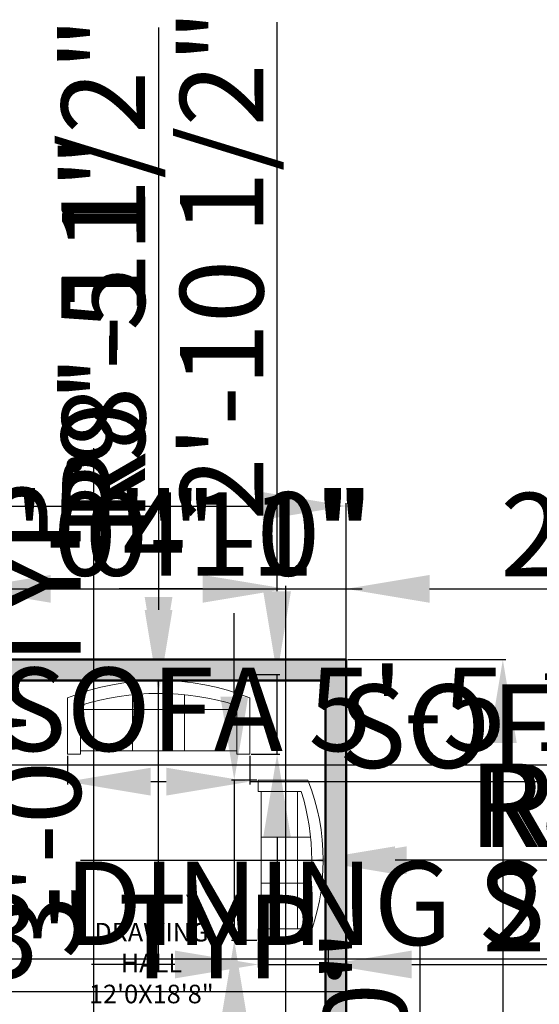
# Model space of a CAD drawing. Units: inches. Extents: x -299 to 1164, y -2 to 940.
# Tile 10 of 11: x 598 to 822, y 490 to 914. Entities that reach past the tile are written whole.
import ezdxf

# ---------------------------------------------------------------- set-up
doc = ezdxf.new("R2010")
doc.units = ezdxf.units.IN
for name, color, linetype, lineweight in [('A-AREA-IDEN', 3, 'Continuous', 25), ('A-FURN', 8, 'Continuous', 18), ('dimensions', 191, 'Continuous', 18), ('outer walls', 7, 'Continuous', 50)]:
    doc.layers.add(name, color=color, linetype=linetype, lineweight=lineweight)
doc.layers.add('A-WALL-PATT', color=240, linetype='Continuous', lineweight=13, true_color=0xed1f24)
doc.styles.get("Standard").update_dxf_attribs({"font": 'arial.ttf'})
doc.dimstyles.new('ISO-25', dxfattribs={"dimtxt": 36, "dimasz": 36, "dimexe": 1.25, "dimexo": 0.625, "dimtad": 1, "dimlunit": 3, "dimtxsty": 'Standard', "dimcen": 2.5, "dimazin": 0, "dimtfac": 1, "dimtmove": 0, "dimatfit": 3, "dimfxl": 1, "dimarcsym": 0})

# ---------------------------------------------------------------- blocks, each defined once
blk = doc.blocks.new('Sofa - Roundback 7 ft.')
for p, q in [((-12.00002, -32.4421), (-12.00003, -6.5971)), ((11.99997, -32.4421), (11.99998, -6.5971)), ((-36.000027, -34), (-36.000027, -11.4696)), ((-35.999844, -13.3819), (35.9998, -13.3819)), ((35.99998, -34), (35.99998, -11.4696)), ((-36.000027, -32.4421), (35.99998, -32.4421))]:
    blk.add_line(p, q)
for points in [[(-36.000027, -34), (-42.000027, -34), (-42.000027, -8)], [(41.99998, -8), (41.99998, -34), (35.99998, -34)]]:
    blk.add_lwpolyline(points)
for centre, radius, start, end in [((0, -114.25), 114.25, 68.43141, 111.5686), ((-0.00001, -127.1968), 121.1968, 72.72033, 107.2797)]:
    blk.add_arc(centre, radius, start, end)
blk = doc.blocks.new('*D13')
at = {"layer": 'Defpoints', "color": 0, "transparency": 16777216}
for p in [(739.07, 704.71), (259.07, 638.49), (739.07, 638.49)]:
    blk.add_point(p, dxfattribs=at)
at = {"layer": 'dimensions', "color": 0, "lineweight": -2, "transparency": 16777216}
for p, q in [((259.07, 639.11), (259.07, 705.96)), ((739.07, 639.11), (739.07, 705.96)), ((295.07, 704.71), (703.07, 704.71))]:
    blk.add_line(p, q, dxfattribs=at)
at = {"layer": 'dimensions', "color": 0, "transparency": 16777216}
for points in [[(295.07, 710.71), (295.07, 698.71), (259.07, 704.71)], [(703.07, 710.71), (703.07, 698.71), (739.07, 704.71)]]:
    blk.add_solid(points, dxfattribs=at)
at = {"layer": 'dimensions', "color": 0, "transparency": 16777216, "insert": (499.07, 723.71), "char_height": 36, "attachment_point": 5}
blk.add_mtext("40'", dxfattribs=at)
blk = doc.blocks.new('*D14')
at = {"layer": 'Defpoints', "color": 0, "transparency": 16777216}
for p in [(739.07, 638.49), (739.07, 158.49), (806.66, 158.49)]:
    blk.add_point(p, dxfattribs=at)
at = {"layer": 'dimensions', "color": 0, "lineweight": -2, "transparency": 16777216}
for p, q in [((739.7, 638.49), (807.91, 638.49)), ((806.66, 602.49), (806.66, 194.49)), ((739.7, 158.49), (807.91, 158.49))]:
    blk.add_line(p, q, dxfattribs=at)
at = {"layer": 'dimensions', "color": 0, "transparency": 16777216}
for points in [[(800.66, 602.49), (812.66, 602.49), (806.66, 638.49)], [(800.66, 194.49), (812.66, 194.49), (806.66, 158.49)]]:
    blk.add_solid(points, dxfattribs=at)
at = {"layer": 'dimensions', "color": 0, "transparency": 16777216, "insert": (787.65, 398.49), "char_height": 36, "attachment_point": 5, "rotation": 90}
blk.add_mtext("40'", dxfattribs=at)
blk = doc.blocks.new('*D19')
at = {"layer": 'Defpoints', "color": 0, "transparency": 16777216}
for p in [(449.18, 602.94), (514.78, 602.94), (514.78, 593.1)]:
    blk.add_point(p, dxfattribs=at)
at = {"layer": 'dimensions', "color": 0, "lineweight": -2, "transparency": 16777216}
for p, q in [((449.18, 602.31), (449.18, 591.85)), ((514.78, 602.31), (514.78, 591.85)), ((413.18, 593.1), (377.18, 593.1)), ((449.18, 593.1), (514.78, 593.1)), ((550.78, 593.1), (918.34, 593.1))]:
    blk.add_line(p, q, dxfattribs=at)
at = {"layer": 'dimensions', "color": 0, "transparency": 16777216}
for points in [[(413.18, 599.1), (413.18, 587.1), (449.18, 593.1)], [(550.78, 599.1), (550.78, 587.1), (514.78, 593.1)]]:
    blk.add_solid(points, dxfattribs=at)
at = {"layer": 'dimensions', "color": 0, "transparency": 16777216, "insert": (752.56, 612.35), "char_height": 36, "attachment_point": 5}
blk.add_mtext('SOFA 5\'-5 1/2"', dxfattribs=at)
blk = doc.blocks.new('*D21')
at = {"layer": 'Defpoints', "color": 0, "transparency": 16777216}
for p in [(618.72, 597.64), (697.42, 597.64), (697.42, 585.83)]:
    blk.add_point(p, dxfattribs=at)
at = {"layer": 'dimensions', "color": 0, "lineweight": -2, "transparency": 16777216}
for p, q in [((618.72, 597.01), (618.72, 584.58)), ((697.42, 597.01), (697.42, 584.58)), ((654.72, 585.83), (661.42, 585.83)), ((697.42, 585.83), (1064.98, 585.83))]:
    blk.add_line(p, q, dxfattribs=at)
at = {"layer": 'dimensions', "color": 0, "transparency": 16777216}
for points in [[(654.72, 591.83), (654.72, 579.83), (618.72, 585.83)], [(661.42, 591.83), (661.42, 579.83), (697.42, 585.83)]]:
    blk.add_solid(points, dxfattribs=at)
at = {"layer": 'dimensions', "color": 0, "transparency": 16777216, "insert": (899.2, 605.08), "char_height": 36, "attachment_point": 5}
blk.add_mtext('SOFA 6\'-6 1/2"', dxfattribs=at)
blk = doc.blocks.new('*D22')
at = {"layer": 'Defpoints', "color": 0, "transparency": 16777216}
for p in [(697.42, 631.99), (709.22, 631.99), (697.42, 597.64)]:
    blk.add_point(p, dxfattribs=at)
at = {"layer": 'dimensions', "color": 0, "lineweight": -2, "transparency": 16777216}
for p, q in [((709.22, 667.99), (709.22, 913.4)), ((698.04, 631.99), (710.47, 631.99)), ((709.22, 597.64), (709.22, 631.99)), ((698.04, 597.64), (710.47, 597.64)), ((709.22, 561.64), (709.22, 525.64))]:
    blk.add_line(p, q, dxfattribs=at)
at = {"layer": 'dimensions', "color": 0, "transparency": 16777216}
for points in [[(703.22, 667.99), (715.22, 667.99), (709.22, 631.99)], [(703.22, 561.64), (715.22, 561.64), (709.22, 597.64)]]:
    blk.add_solid(points, dxfattribs=at)
at = {"layer": 'dimensions', "color": 0, "transparency": 16777216, "insert": (689.98, 808.7), "char_height": 36, "attachment_point": 5, "rotation": 90}
blk.add_mtext('2\'-10 1/2"', dxfattribs=at)
blk = doc.blocks.new('*D23')
at = {"layer": 'Defpoints', "color": 0, "transparency": 16777216}
for p in [(701.12, 586.52), (690.74, 517.34), (701.12, 517.34)]:
    blk.add_point(p, dxfattribs=at)
at = {"layer": 'dimensions', "color": 0, "lineweight": -2, "transparency": 16777216}
for p, q in [((690.74, 622.52), (690.74, 658.52)), ((700.49, 586.52), (689.49, 586.52)), ((690.74, 586.52), (690.74, 517.34)), ((700.49, 517.34), (689.49, 517.34)), ((690.74, 481.34), (690.74, 197.66))]:
    blk.add_line(p, q, dxfattribs=at)
at = {"layer": 'dimensions', "color": 0, "transparency": 16777216}
for points in [[(684.74, 622.52), (696.74, 622.52), (690.74, 586.52)], [(684.74, 481.34), (696.74, 481.34), (690.74, 517.34)]]:
    blk.add_solid(points, dxfattribs=at)
at = {"layer": 'dimensions', "color": 0, "transparency": 16777216, "insert": (671.49, 321.5), "char_height": 36, "attachment_point": 5, "rotation": 90}
blk.add_mtext('SOFA 5\'-9"', dxfattribs=at)
blk = doc.blocks.new('*D24')
at = {"layer": 'Defpoints', "color": 0, "transparency": 16777216}
for p in [(701.12, 517.34), (731.32, 517.34), (731.32, 506.96)]:
    blk.add_point(p, dxfattribs=at)
at = {"layer": 'dimensions', "color": 0, "lineweight": -2, "transparency": 16777216}
for p, q in [((701.12, 516.71), (701.12, 505.71)), ((731.32, 516.71), (731.32, 505.71)), ((665.12, 506.96), (629.12, 506.96)), ((701.12, 506.96), (731.32, 506.96)), ((767.32, 506.96), (900.88, 506.96))]:
    blk.add_line(p, q, dxfattribs=at)
at = {"layer": 'dimensions', "color": 0, "transparency": 16777216}
for points in [[(665.12, 512.96), (665.12, 500.96), (701.12, 506.96)], [(767.32, 512.96), (767.32, 500.96), (731.32, 506.96)]]:
    blk.add_solid(points, dxfattribs=at)
at = {"layer": 'dimensions', "color": 0, "transparency": 16777216, "insert": (852.1, 525.97), "char_height": 36, "attachment_point": 5}
blk.add_mtext('2\'-6"', dxfattribs=at)
blk = doc.blocks.new('*D35')
at = {"layer": 'Defpoints', "color": 0, "transparency": 16777216}
for p in [(307.07, 495.34), (268.07, 489.49), (307.07, 489.49)]:
    blk.add_point(p, dxfattribs=at)
at = {"layer": 'dimensions', "color": 0, "lineweight": -2, "transparency": 16777216}
for p, q in [((232.07, 495.34), (196.07, 495.34)), ((268.07, 490.11), (268.07, 496.59)), ((268.07, 495.34), (307.07, 495.34)), ((307.07, 490.11), (307.07, 496.59)), ((343.07, 495.34), (749.73, 495.34))]:
    blk.add_line(p, q, dxfattribs=at)
at = {"layer": 'dimensions', "color": 0, "transparency": 16777216}
for points in [[(232.07, 501.34), (232.07, 489.34), (268.07, 495.34)], [(343.07, 501.34), (343.07, 489.34), (307.07, 495.34)]]:
    blk.add_solid(points, dxfattribs=at)
at = {"layer": 'dimensions', "color": 0, "transparency": 16777216, "insert": (564.4, 514.36), "char_height": 36, "attachment_point": 5}
blk.add_mtext('VENT 3\'-3" TYP.', dxfattribs=at)
blk = doc.blocks.new('*D37')
at = {"layer": 'Defpoints', "color": 0, "transparency": 16777216}
for p in [(588.07, 400.99), (624.7, 400.99), (624.7, 395.5)]:
    blk.add_point(p, dxfattribs=at)
at = {"layer": 'dimensions', "color": 0, "lineweight": -2, "transparency": 16777216}
for p, q in [((588.07, 400.36), (588.07, 394.25)), ((624.7, 400.36), (624.7, 394.25)), ((552.07, 395.5), (516.07, 395.5)), ((588.07, 395.5), (624.7, 395.5)), ((660.7, 395.5), (1164.33, 395.5))]:
    blk.add_line(p, q, dxfattribs=at)
at = {"layer": 'dimensions', "color": 0, "transparency": 16777216}
for points in [[(552.07, 401.5), (552.07, 389.5), (588.07, 395.5)], [(660.7, 401.5), (660.7, 389.5), (624.7, 395.5)]]:
    blk.add_solid(points, dxfattribs=at)
at = {"layer": 'dimensions', "color": 0, "transparency": 16777216, "insert": (930.51, 414.76), "char_height": 36, "attachment_point": 5}
blk.add_mtext('DOOR 3\'-0 1/2" TYP.', dxfattribs=at)
blk = doc.blocks.new('*D38')
at = {"layer": 'Defpoints', "color": 0, "transparency": 16777216}
for p in [(624.7, 437.08), (630.19, 437.08), (624.7, 400.99)]:
    blk.add_point(p, dxfattribs=at)
at = {"layer": 'dimensions', "color": 0, "lineweight": -2, "transparency": 16777216}
for p, q in [((630.19, 473.08), (630.19, 729.74)), ((625.32, 437.08), (631.44, 437.08)), ((630.19, 400.99), (630.19, 437.08)), ((625.32, 400.99), (631.44, 400.99)), ((630.19, 364.99), (630.19, 328.99))]:
    blk.add_line(p, q, dxfattribs=at)
at = {"layer": 'dimensions', "color": 0, "transparency": 16777216}
for points in [[(624.19, 473.08), (636.19, 473.08), (630.19, 437.08)], [(624.19, 364.99), (636.19, 364.99), (630.19, 400.99)]]:
    blk.add_solid(points, dxfattribs=at)
at = {"layer": 'dimensions', "color": 0, "transparency": 16777216, "insert": (611.17, 619.41), "char_height": 36, "attachment_point": 5, "rotation": 90}
blk.add_mtext('3\'-0" TYP.', dxfattribs=at)
blk = doc.blocks.new('*D39')
at = {"layer": 'Defpoints', "color": 0, "transparency": 16777216}
for p in [(575.6, 509.45), (484.6, 495.8), (575.6, 495.8)]:
    blk.add_point(p, dxfattribs=at)
at = {"layer": 'dimensions', "color": 0, "lineweight": -2, "transparency": 16777216}
for p, q in [((484.6, 496.43), (484.6, 510.7)), ((575.6, 496.43), (575.6, 510.7)), ((520.6, 509.45), (539.6, 509.45)), ((575.6, 509.45), (1008.53, 509.45))]:
    blk.add_line(p, q, dxfattribs=at)
at = {"layer": 'dimensions', "color": 0, "transparency": 16777216}
for points in [[(520.6, 515.45), (520.6, 503.45), (484.6, 509.45)], [(539.6, 515.45), (539.6, 503.45), (575.6, 509.45)]]:
    blk.add_solid(points, dxfattribs=at)
at = {"layer": 'dimensions', "color": 0, "transparency": 16777216, "insert": (810.07, 528.69), "char_height": 36, "attachment_point": 5}
blk.add_mtext('DINING SET 7\'-7"', dxfattribs=at)
blk = doc.blocks.new('*D47')
at = {"layer": 'Defpoints', "color": 0, "transparency": 16777216}
for p in [(502.07, 668.99), (466.07, 222.49), (502.07, 222.49)]:
    blk.add_point(p, dxfattribs=at)
at = {"layer": 'dimensions', "color": 0, "lineweight": -2, "transparency": 16777216}
for p, q in [((430.07, 668.99), (394.07, 668.99)), ((466.07, 223.11), (466.07, 670.24)), ((466.07, 668.99), (502.07, 668.99)), ((502.07, 223.11), (502.07, 670.24)), ((538.07, 668.99), (670.99, 668.99))]:
    blk.add_line(p, q, dxfattribs=at)
at = {"layer": 'dimensions', "color": 0, "transparency": 16777216}
for points in [[(430.07, 674.99), (430.07, 662.99), (466.07, 668.99)], [(538.07, 674.99), (538.07, 662.99), (502.07, 668.99)]]:
    blk.add_solid(points, dxfattribs=at)
at = {"layer": 'dimensions', "color": 0, "transparency": 16777216, "insert": (622.53, 688.01), "char_height": 36, "attachment_point": 5}
blk.add_mtext('3\'-0"', dxfattribs=at)
blk = doc.blocks.new('*D48')
at = {"layer": 'Defpoints', "color": 0, "transparency": 16777216}
for p in [(546.07, 668.99), (535.07, 222.49), (546.07, 222.49)]:
    blk.add_point(p, dxfattribs=at)
at = {"layer": 'dimensions', "color": 0, "lineweight": -2, "transparency": 16777216}
for p, q in [((499.07, 668.99), (463.07, 668.99)), ((535.07, 223.11), (535.07, 670.24)), ((535.07, 668.99), (546.07, 668.99)), ((546.07, 223.11), (546.07, 670.24)), ((582.07, 668.99), (742.99, 668.99))]:
    blk.add_line(p, q, dxfattribs=at)
at = {"layer": 'dimensions', "color": 0, "transparency": 16777216}
for points in [[(499.07, 674.99), (499.07, 662.99), (535.07, 668.99)], [(582.07, 674.99), (582.07, 662.99), (546.07, 668.99)]]:
    blk.add_solid(points, dxfattribs=at)
at = {"layer": 'dimensions', "color": 0, "transparency": 16777216, "insert": (680.53, 687.99), "char_height": 36, "attachment_point": 5}
blk.add_mtext('0\'-11"', dxfattribs=at)
blk = doc.blocks.new('*D51')
at = {"layer": 'Defpoints', "color": 0, "transparency": 16777216}
for p in [(739.07, 668.99), (713.07, 405.49), (739.07, 396.49)]:
    blk.add_point(p, dxfattribs=at)
at = {"layer": 'dimensions', "color": 0, "lineweight": -2, "transparency": 16777216}
for p, q in [((677.07, 668.99), (641.07, 668.99)), ((713.07, 406.11), (713.07, 670.24)), ((713.07, 668.99), (739.07, 668.99)), ((739.07, 397.11), (739.07, 670.24)), ((775.07, 668.99), (908.63, 668.99))]:
    blk.add_line(p, q, dxfattribs=at)
at = {"layer": 'dimensions', "color": 0, "transparency": 16777216}
for points in [[(677.07, 674.99), (677.07, 662.99), (713.07, 668.99)], [(775.07, 674.99), (775.07, 662.99), (739.07, 668.99)]]:
    blk.add_solid(points, dxfattribs=at)
at = {"layer": 'dimensions', "color": 0, "transparency": 16777216, "insert": (859.85, 687.69), "char_height": 36, "attachment_point": 5}
blk.add_mtext('2\'-2"', dxfattribs=at)
blk = doc.blocks.new('*D52')
at = {"layer": 'Defpoints', "color": 0, "transparency": 16777216}
for p in [(575.54, 668.99), (527.54, 311.49), (575.54, 311.49)]:
    blk.add_point(p, dxfattribs=at)
at = {"layer": 'dimensions', "color": 0, "lineweight": -2, "transparency": 16777216}
for p, q in [((491.54, 668.99), (455.54, 668.99)), ((527.54, 312.11), (527.54, 670.24)), ((527.54, 668.99), (575.54, 668.99)), ((575.54, 312.11), (575.54, 670.24)), ((611.54, 668.99), (745.94, 668.99))]:
    blk.add_line(p, q, dxfattribs=at)
at = {"layer": 'dimensions', "color": 0, "transparency": 16777216}
for points in [[(491.54, 674.99), (491.54, 662.99), (527.54, 668.99)], [(611.54, 674.99), (611.54, 662.99), (575.54, 668.99)]]:
    blk.add_solid(points, dxfattribs=at)
at = {"layer": 'dimensions', "color": 0, "transparency": 16777216, "insert": (696.74, 687.99), "char_height": 36, "attachment_point": 5}
blk.add_mtext('4\'-0"', dxfattribs=at)
blk = doc.blocks.new('*D58')
at = {"layer": 'Defpoints', "color": 0, "transparency": 16777216}
for p in [(456.35, 347.49), (770.93, 347.49), (456.35, 311.49)]:
    blk.add_point(p, dxfattribs=at)
at = {"layer": 'dimensions', "color": 0, "lineweight": -2, "transparency": 16777216}
for p, q in [((770.93, 383.49), (770.93, 516.41)), ((456.97, 347.49), (772.18, 347.49)), ((770.93, 311.49), (770.93, 347.49)), ((456.97, 311.49), (772.18, 311.49)), ((770.93, 275.49), (770.93, 239.49))]:
    blk.add_line(p, q, dxfattribs=at)
at = {"layer": 'dimensions', "color": 0, "transparency": 16777216}
for points in [[(764.93, 383.49), (776.93, 383.49), (770.93, 347.49)], [(764.93, 275.49), (776.93, 275.49), (770.93, 311.49)]]:
    blk.add_solid(points, dxfattribs=at)
at = {"layer": 'dimensions', "color": 0, "transparency": 16777216, "insert": (751.91, 467.95), "char_height": 36, "attachment_point": 5, "rotation": 90}
blk.add_mtext('3\'-0"', dxfattribs=at)
blk = doc.blocks.new('*D63')
at = {"layer": 'Defpoints', "color": 0, "transparency": 16777216}
for p in [(658.07, 623.87), (658.07, 510.33)]:
    blk.add_point(p, dxfattribs=at)
at = {"layer": 'dimensions', "color": 0, "lineweight": -2, "transparency": 16777216}
for p, q in [((658.07, 911.15), (658.07, 659.87)), ((658.07, 510.33), (658.07, 623.87))]:
    blk.add_line(p, q, dxfattribs=at)
at = {"layer": 'dimensions', "color": 0, "transparency": 16777216}
blk.add_solid([(652.07, 659.87), (664.07, 659.87), (658.07, 623.87)], dxfattribs=at)
at = {"layer": 'dimensions', "color": 0, "transparency": 16777216, "insert": (638.83, 803.51), "char_height": 36, "attachment_point": 5, "rotation": 90}
blk.add_mtext('R9\'-5 1/2"', dxfattribs=at)
blk = doc.blocks.new('*D64')
at = {"layer": 'Defpoints', "color": 0, "transparency": 16777216}
for p in [(658.07, 629.49), (658.07, 522.46)]:
    blk.add_point(p, dxfattribs=at)
at = {"layer": 'dimensions', "color": 0, "lineweight": -2, "transparency": 16777216}
for p, q in [((658.07, 860.86), (658.07, 665.49)), ((658.07, 522.46), (658.07, 629.49))]:
    blk.add_line(p, q, dxfattribs=at)
at = {"layer": 'dimensions', "color": 0, "transparency": 16777216}
blk.add_solid([(652.07, 665.49), (664.07, 665.49), (658.07, 629.49)], dxfattribs=at)
at = {"layer": 'dimensions', "color": 0, "transparency": 16777216, "insert": (639.07, 781.17), "char_height": 36, "attachment_point": 5, "rotation": 90}
blk.add_mtext('R8\'-11"', dxfattribs=at)
blk = doc.blocks.new('*D65')
at = {"layer": 'Defpoints', "color": 0, "transparency": 16777216}
for p in [(624.36, 551.93), (724.18, 551.93)]:
    blk.add_point(p, dxfattribs=at)
at = {"layer": 'dimensions', "color": 0, "lineweight": -2, "transparency": 16777216}
for p, q in [((624.36, 551.93), (724.18, 551.93)), ((927.58, 551.93), (760.18, 551.93))]:
    blk.add_line(p, q, dxfattribs=at)
at = {"layer": 'dimensions', "color": 0, "transparency": 16777216}
blk.add_solid([(760.18, 557.93), (760.18, 545.93), (724.18, 551.93)], dxfattribs=at)
at = {"layer": 'dimensions', "color": 0, "transparency": 16777216, "insert": (861.88, 570.93), "char_height": 36, "attachment_point": 5, "rotation": 0.0001}
blk.add_mtext('R8\'-4"', dxfattribs=at)
blk = doc.blocks.new('*D66')
at = {"layer": 'Defpoints', "color": 0, "transparency": 16777216}
for p in [(635.03, 551.93), (729.12, 551.93)]:
    blk.add_point(p, dxfattribs=at)
at = {"layer": 'dimensions', "color": 0, "lineweight": -2, "transparency": 16777216}
for p, q in [((635.03, 551.93), (729.12, 551.93)), ((960.49, 551.93), (765.12, 551.93))]:
    blk.add_line(p, q, dxfattribs=at)
at = {"layer": 'dimensions', "color": 0, "transparency": 16777216}
blk.add_solid([(765.12, 557.93), (765.12, 545.93), (729.12, 551.93)], dxfattribs=at)
at = {"layer": 'dimensions', "color": 0, "transparency": 16777216, "insert": (880.81, 570.93), "char_height": 36, "attachment_point": 5, "rotation": 0.0001}
blk.add_mtext('R7\'-10"', dxfattribs=at)

msp = doc.modelspace()

# ---------------------------------------------------------------- hatches: boundary and pattern name
at = {"layer": 'A-WALL-PATT'}
h = msp.add_hatch(color=256, dxfattribs=at)
h.dxf.hatch_style = 1
h.paths.add_polyline_path([(312.071, 460.489), (307.071, 460.489), (307.071, 432.489), (307.071, 427.489), (372.071, 427.489), (372.071, 375.489), (372.071, 370.489), (380.071, 370.489, -0.0217424), (380.071, 372.989), (380.071, 375.489), (377.071, 375.489), (377.071, 427.489), (417.071, 427.489), (417.071, 489.489), (412.071, 489.489), (412.071, 484.489), (412.071, 432.489), (312.071, 432.489)], flags=17)
h.paths.add_polyline_path([(340.071, 372.989, -0.0217424), (340.071, 375.489), (268.071, 375.489), (268.071, 427.489), (268.071, 432.489), (268.071, 484.489), (268.071, 489.489), (268.071, 629.489), (412.071, 629.489), (412.071, 527.563, -0.0185322), (414.571, 527.489), (417.071, 527.489), (417.071, 629.489), (581.071, 629.489), (581.071, 553.489), (586.071, 553.489), (586.071, 629.489), (730.071, 629.489), (730.071, 405.489), (713.071, 405.489), (713.071, 396.489), (739.071, 396.489), (739.071, 638.489), (259.071, 638.489), (259.071, 183.489), (304.071, 183.489), (304.071, 192.489), (268.071, 192.489), (268.071, 370.489), (340.071, 370.489)])
h.paths.add_polyline_path([(417.071, 188.489), (417.071, 213.489), (461.071, 213.489), (461.071, 188.489)], flags=16)
h.paths.add_polyline_path([(586.071, 313.578), (577.071, 313.578), (577.071, 311.489), (575.54, 311.489), (575.54, 302.489), (586.071, 302.489)], flags=16)
h.paths.add_polyline_path([(586.071, 405.489), (586.071, 481.489), (581.071, 481.489), (581.071, 432.489), (499.071, 432.489), (499.071, 427.489), (577.071, 427.489), (577.071, 385.578), (586.071, 385.578), (586.071, 396.489)], flags=17)
h.paths.add_polyline_path([(641.071, 405.489), (624.071, 405.489, -0.0333689), (624.071, 400.989), (624.071, 396.489), (641.071, 396.489)], flags=17)
h.paths.add_polyline_path([(491.866, 222.489), (491.866, 213.489), (586.071, 213.489), (586.071, 222.489)])
edge = h.paths.add_edge_path()
edge.add_line((467.866, 213.489), (467.866, 222.489))
edge.add_line((467.866, 222.489), (466.071, 222.489))
edge.add_line((466.071, 222.489), (466.071, 302.489))
edge.add_line((466.071, 302.489), (527.54, 302.489))
edge.add_line((527.54, 302.489), (527.54, 311.489))
edge.add_line((527.54, 311.489), (449.071, 311.489))
edge.add_line((449.071, 311.489), (449.071, 308.989))
edge.add_arc((420.339, 307.739), 28.759, -2.4911, 2.4911, ccw=False)
edge.add_line((449.071, 306.489), (461.071, 306.489))
edge.add_line((461.071, 306.489), (461.071, 222.489))
edge.add_line((461.071, 222.489), (443.844, 222.489))
edge.add_line((443.844, 222.489), (443.844, 213.489))
edge.add_line((443.844, 213.489), (419.844, 213.489))
edge.add_line((419.844, 213.489), (419.844, 222.489))
edge.add_line((419.844, 222.489), (417.071, 222.489))
edge.add_line((417.071, 222.489), (417.071, 306.489))
edge.add_line((417.071, 306.489), (417.071, 311.489))
edge.add_line((417.071, 311.489), (417.071, 375.489))
edge.add_line((417.071, 375.489), (412.071, 375.489))
edge.add_line((412.071, 375.489), (412.071, 370.489))
edge.add_line((412.071, 370.489), (412.071, 192.489))
edge.add_line((412.071, 192.489), (376.071, 192.489))
edge.add_line((376.071, 192.489), (376.071, 183.489))
edge.add_line((376.071, 183.489), (412.071, 183.489))
edge.add_line((412.071, 183.489), (466.071, 183.489))
edge.add_line((466.071, 183.489), (466.071, 213.489))
edge.add_line((466.071, 213.489), (467.866, 213.489))

# ---------------------------------------------------------------- linework, layer by layer
at = {"layer": 'outer walls'}
for p, q in [((739.071, 638.489), (259.071, 638.489)), ((739.071, 158.489), (739.071, 638.489)), ((730.071, 629.489), (586.071, 629.489)), ((730.071, 405.489), (730.071, 629.489))]:
    msp.add_line(p, q, dxfattribs=at)

# ---------------------------------------------------------------- block references
at = {"layer": 'A-FURN', "xscale": 0.9368190995228506, "yscale": 0.9368190995228506, "zscale": 0.9368190995228506}
msp.add_blockref('Sofa - Roundback 7 ft.', (658.071, 629.489), dxfattribs=at)
at = {"layer": 'A-FURN', "xscale": 0.8235785891221066, "yscale": 0.8235785891221066, "zscale": 0.8235785891221066, "rotation": 270}
msp.add_blockref('Sofa - Roundback 7 ft.', (729.12, 551.928), dxfattribs=at)

# ---------------------------------------------------------------- texts
at = {"layer": 'A-AREA-IDEN', "insert": (620.054, 524.904), "char_height": 8, "attachment_point": 1}
msp.add_mtext_dynamic_manual_height_columns('\\pxqc,t15;DRAWING HALL\\P12\'0X18\'8"', width=69.83809, gutter_width=12.5, heights=[0], dxfattribs=at)

# ---------------------------------------------------------------- dimensions: what is measured, and where the dimension line sits
at = {"layer": 'dimensions'}
for base, p1, p2, override, picture, middle in [((709.22139, 631.98722), (697.41747, 597.63718), (697.41747, 631.98722), {"dimdec": 1, "dimlfac": 1, "dimrnd": 0, "dimzin": 1, "dimdsep": 46, "dimlunit": 4, "dimfrac": 2}, '*D22', (689.98248, 808.69544)), ((806.659, 158.489), (739.071, 638.489), (739.071, 158.489), {"dimclrd": 0, "dimclre": 0, "dimclrt": 0}, '*D14', (787.654, 398.489)), ((770.929, 347.489), (456.348, 311.489), (456.348, 347.489), {"dimdec": 1, "dimlfac": 1, "dimrnd": 0, "dimzin": 1, "dimdsep": 46, "dimlunit": 4, "dimfrac": 2}, '*D58', (751.911, 467.95))]:
    dim = msp.add_linear_dim(base=base, p1=p1, p2=p2, angle=90, dimstyle='ISO-25', override=override, dxfattribs=at)
    dim.commit()
    dim.dimension.update_dxf_attribs({"geometry": picture, "text_midpoint": middle})
for center, mpoint, picture, middle in [((658.071, 510.329), (658.071, 623.868), '*D63', (638.832, 803.511)), ((658.071, 522.457), (658.071, 629.489), '*D64', (639.065, 781.174)), ((624.364, 551.928), (724.179, 551.928), '*D65', (861.879, 570.934)), ((635.027, 551.928), (729.12, 551.928), '*D66', (880.805, 570.934))]:
    dim = msp.add_radius_dim(center=center, mpoint=mpoint, dimstyle='ISO-25', override={"dimdec": 1, "dimlfac": 1, "dimrnd": 0, "dimzin": 1, "dimdsep": 46, "dimlunit": 4, "dimfrac": 2}, dxfattribs=at)
    dim.commit()
    dim.dimension.update_dxf_attribs({"geometry": picture, "text_midpoint": middle})
for base, p1, p2, override, picture, middle in [((739.071, 704.705), (259.071, 638.489), (739.071, 638.489), {"dimclrd": 0, "dimclre": 0, "dimclrt": 0}, '*D13', (499.071, 723.711)), ((502.071, 668.989), (466.071, 222.489), (502.071, 222.489), {"dimdec": 1, "dimlfac": 1, "dimrnd": 0, "dimzin": 1, "dimdsep": 46, "dimlunit": 4, "dimfrac": 2}, '*D47', (622.532, 688.007)), ((575.54, 668.989), (527.54, 311.489), (575.54, 311.489), {"dimdec": 1, "dimlfac": 1, "dimrnd": 0, "dimzin": 1, "dimdsep": 46, "dimlunit": 4, "dimfrac": 2}, '*D52', (696.738, 687.995)), ((546.071, 668.989), (535.071, 222.489), (546.071, 222.489), {"dimdec": 1, "dimlfac": 1, "dimrnd": 0, "dimzin": 1, "dimdsep": 46, "dimlunit": 4, "dimfrac": 2}, '*D48', (680.53, 687.995)), ((739.071, 668.989), (713.071, 405.489), (739.071, 396.489), {"dimdec": 1, "dimlfac": 1, "dimrnd": 0, "dimzin": 1, "dimdsep": 46, "dimlunit": 4, "dimfrac": 2}, '*D51', (859.852, 687.688)), ((731.317, 506.96), (701.119, 517.338), (731.317, 517.338), {"dimdec": 1, "dimlfac": 1, "dimrnd": 0, "dimzin": 1, "dimdsep": 46, "dimlunit": 4, "dimfrac": 2}, '*D24', (852.097, 525.966))]:
    dim = msp.add_linear_dim(base=base, p1=p1, p2=p2, dimstyle='ISO-25', override=override, dxfattribs=at)
    dim.commit()
    dim.dimension.update_dxf_attribs({"geometry": picture, "text_midpoint": middle})
for base, p1, p2, angle, text, picture, middle in [((630.192, 437.079), (624.698, 400.989), (624.698, 437.079), 90, '<> TYP.', '*D38', (611.174, 619.411)), ((690.742, 517.338), (701.119, 586.518), (701.119, 517.338), 270, 'SOFA <>', '*D23', (671.49, 321.5))]:
    dim = msp.add_linear_dim(base=base, p1=p1, p2=p2, angle=angle, text=text, dimstyle='ISO-25', override={"dimdec": 1, "dimlfac": 1, "dimrnd": 0, "dimzin": 1, "dimdsep": 46, "dimlunit": 4, "dimfrac": 2}, dxfattribs=at)
    dim.commit()
    dim.dimension.update_dxf_attribs({"geometry": picture, "text_midpoint": middle})
for base, p1, p2, text, picture, middle in [((514.778, 593.095), (449.176, 602.936), (514.778, 602.936), 'SOFA <>', '*D19', (752.559, 612.347)), ((697.417, 585.833), (618.725, 597.637), (697.417, 597.637), 'SOFA <>', '*D21', (899.198, 605.084)), ((575.6, 509.45), (484.6, 495.8), (575.6, 495.8), 'DINING SET <>', '*D39', (810.066, 528.689)), ((307.071, 495.339), (268.071, 489.489), (307.071, 489.489), 'VENT <> TYP.', '*D35', (564.399, 514.357)), ((624.698, 395.495), (588.071, 400.989), (624.698, 400.989), 'DOOR <> TYP.', '*D37', (930.512, 414.759))]:
    dim = msp.add_linear_dim(base=base, p1=p1, p2=p2, text=text, dimstyle='ISO-25', override={"dimdec": 1, "dimlfac": 1, "dimrnd": 0, "dimzin": 1, "dimdsep": 46, "dimlunit": 4, "dimfrac": 2}, dxfattribs=at)
    dim.commit()
    dim.dimension.update_dxf_attribs({"geometry": picture, "text_midpoint": middle})

doc.saveas('drawing.dxf')
